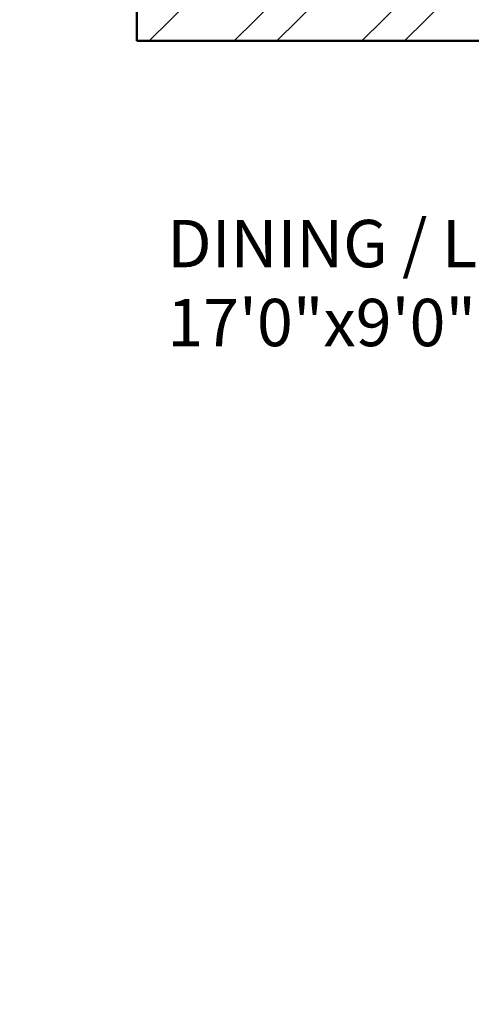
# Model space of a CAD drawing. Units: inches. Extents: x 963 to 2075, y 289 to 2657.
# Tile 89 of 98: x 1681 to 1728, y 2221 to 2325. Entities that reach past the tile are written whole.
import ezdxf

# ---------------------------------------------------------------- set-up
doc = ezdxf.new("R2010")
doc.units = ezdxf.units.IN
for name, color, linetype, lineweight in [('A-AREA-IDEN', 7, 'Continuous', 18), ('A-WALL', 7, 'Continuous', 50), ('A-WALL-PATT', 8, 'Continuous', 13)]:
    doc.layers.add(name, color=color, linetype=linetype, lineweight=lineweight)
doc.styles.get("Standard").update_dxf_attribs({"font": 'arial.ttf'})

msp = doc.modelspace()

# ---------------------------------------------------------------- hatches: boundary and pattern name
at = {"layer": 'A-WALL-PATT'}
h = msp.add_hatch(dxfattribs=at)
h.set_pattern_fill('ANSI32', color=256)
h.paths.add_polyline_path([(1296.92, 2558.32), (1203.92, 2558.32), (1203.92, 2493.82), (1191.53, 2493.82), (1191.53, 2489.32), (1211.06, 2489.32), (1211.06, 2492.02), (1211.06, 2493.82), (1208.42, 2493.82), (1208.42, 2553.82), (1292.42, 2553.82), (1292.42, 2538.86), (1296.92, 2538.86)])
h.paths.add_polyline_path([(1442.42, 2558.32), (1349.42, 2558.32), (1349.42, 2538.94), (1353.92, 2538.94), (1353.92, 2553.82), (1437.92, 2553.82), (1437.92, 2493.82), (1434.54, 2493.82), (1434.54, 2489.32), (1448.31, 2489.32), (1448.31, 2491.57), (1448.31, 2493.82), (1442.42, 2493.82)])
h.paths.add_polyline_path([(1415.55, 2491.57), (1415.55, 2493.82), (1340.94, 2493.82), (1340.94, 2489.32), (1371.92, 2489.32), (1371.92, 2378.32), (1367.6, 2378.32), (1367.6, 2373.82), (1371.92, 2373.82), (1371.92, 2355.19), (1376.42, 2355.19), (1376.42, 2489.32), (1415.55, 2489.32)])
h.paths.add_polyline_path([(1304.94, 2491.57), (1304.94, 2493.82), (1296.92, 2493.82), (1296.92, 2514.86), (1292.42, 2514.86), (1292.42, 2493.82), (1232.81, 2493.82), (1232.81, 2489.32), (1256.42, 2489.32), (1256.42, 2327.32), (1253.71, 2327.32), (1253.71, 2322.82), (1328.42, 2322.82), (1328.42, 2331.15), (1323.92, 2331.15), (1323.92, 2327.32), (1260.92, 2327.32), (1260.92, 2373.82), (1323.92, 2373.82), (1323.92, 2357.81), (1328.42, 2357.81), (1328.42, 2373.82), (1346.01, 2373.82), (1346.01, 2376.07), (1346.01, 2378.32), (1260.92, 2378.32), (1260.92, 2489.32), (1304.94, 2489.32)])
h.paths.add_polyline_path([(1226.65, 2327.32), (1124.42, 2327.32), (1124.42, 2347.45), (1119.92, 2347.45), (1119.92, 2322.82), (1163.42, 2322.82), (1163.42, 2305.43), (1165.67, 2305.43), (1167.92, 2305.43), (1167.92, 2322.82), (1226.65, 2322.82), (1226.65, 2325.07)])
h.paths.add_polyline_path([(1095.92, 2489.32), (1124.42, 2489.32), (1131.53, 2489.32), (1131.53, 2491.57), (1131.53, 2493.82), (1119.92, 2493.82), (1091.42, 2493.82), (1091.42, 2417.32), (1095.92, 2417.32), (1119.92, 2417.32), (1119.92, 2407.45), (1124.42, 2407.45), (1124.42, 2421.82), (1095.92, 2421.82)])
h.paths.add_polyline_path([(1512.92, 2558.32), (1508.42, 2558.32), (1508.42, 2493.82), (1503.4, 2493.82), (1503.4, 2489.32), (1508.42, 2489.32), (1508.42, 2327.32), (1376.42, 2327.32), (1376.42, 2330.27), (1371.92, 2330.27), (1371.92, 2298.74), (1376.42, 2298.74), (1376.42, 2322.82), (1508.42, 2322.82), (1508.42, 2165.32), (1504.26, 2165.32), (1504.26, 2160.82), (1508.42, 2160.82), (1508.42, 2108.32), (1512.92, 2108.32), (1512.92, 2160.82), (1516.18, 2160.82), (1516.18, 2163.07), (1516.18, 2165.32), (1512.92, 2165.32), (1512.92, 2322.82), (1644.92, 2322.82), (1644.92, 2298.74), (1649.42, 2298.74), (1649.42, 2322.82), (1649.42, 2330.94), (1647.17, 2330.94), (1644.92, 2330.94), (1644.92, 2327.32), (1512.92, 2327.32), (1512.92, 2489.32), (1516.76, 2489.32), (1516.76, 2491.57), (1516.76, 2493.82), (1512.92, 2493.82)])
h.paths.add_polyline_path([(1671.92, 2558.32), (1578.92, 2558.32), (1578.92, 2493.82), (1573.53, 2493.82), (1573.53, 2489.32), (1586.54, 2489.32), (1586.54, 2491.57), (1586.54, 2493.82), (1583.42, 2493.82), (1583.42, 2553.82), (1667.42, 2553.82), (1667.42, 2541.11), (1671.92, 2541.11)])
h.paths.add_polyline_path([(1681.26, 2493.82), (1671.92, 2493.82), (1671.92, 2517.11), (1667.42, 2517.11), (1667.42, 2493.82), (1610.22, 2493.82), (1610.22, 2489.32), (1644.92, 2489.32), (1644.92, 2357.87), (1649.42, 2357.87), (1649.42, 2373.82), (1652.2, 2373.82), (1652.2, 2375.83), (1652.2, 2378.32), (1649.42, 2378.32), (1649.42, 2489.32), (1681.26, 2489.32), (1681.26, 2491.57)])
h.paths.add_polyline_path([(1821.92, 2558.32), (1728.92, 2558.32), (1728.92, 2541), (1733.42, 2541), (1733.42, 2553.82), (1817.42, 2553.82), (1817.42, 2493.82), (1813.51, 2493.82), (1813.51, 2489.32), (1830.08, 2489.32), (1830.08, 2491.57), (1830.08, 2493.82), (1821.92, 2493.82)])
h.paths.add_polyline_path([(1794.24, 2493.82), (1717.26, 2493.82), (1717.26, 2489.32), (1760.42, 2489.32), (1760.42, 2378.32), (1674.4, 2378.32), (1674.4, 2373.82), (1692.92, 2373.82), (1692.92, 2356.95), (1697.42, 2356.95), (1697.42, 2373.82), (1760.42, 2373.82), (1760.42, 2327.32), (1697.42, 2327.32), (1697.42, 2333.34), (1692.92, 2333.34), (1692.92, 2322.82), (1768.04, 2322.82), (1768.04, 2325.07), (1768.04, 2327.32), (1764.92, 2327.32), (1764.92, 2489.32), (1794.24, 2489.32)])
h.paths.add_polyline_path([(1733.42, 2517), (1728.92, 2517), (1728.92, 2493.82), (1733.42, 2493.82)], flags=17)
h.paths.add_polyline_path([(1929.92, 2493.82), (1890.08, 2493.82), (1890.08, 2489.32), (1896.92, 2489.32), (1925.42, 2489.32), (1925.42, 2421.82), (1896.92, 2421.82), (1896.92, 2408.32), (1901.42, 2408.32), (1901.42, 2417.32), (1925.42, 2417.32), (1929.92, 2417.32)])
h.paths.add_polyline_path([(1901.42, 2348.32), (1896.92, 2348.32), (1896.92, 2327.32), (1800.42, 2327.32), (1800.42, 2322.82), (1853.42, 2322.82), (1853.42, 2309.45), (1857.92, 2309.45), (1857.92, 2322.82), (1901.42, 2322.82)])
h.paths.add_polyline_path([(1857.92, 2249.45), (1853.42, 2249.45), (1853.42, 2214.82), (1686.31, 2214.82), (1686.31, 2210.32), (1853.42, 2210.32), (1853.42, 2202.13), (1857.92, 2202.13), (1857.92, 2210.32)])
h.paths.add_polyline_path([(1857.92, 2142.13), (1853.42, 2142.13), (1853.42, 2115.42), (1841.42, 2115.42), (1841.42, 2088.53), (1841.42, 2046.95), (1845.92, 2046.95), (1845.92, 2110.92), (1905.92, 2110.92), (1905.92, 2092.52), (1910.42, 2092.52), (1910.42, 2115.42), (1857.92, 2115.42)])
h.paths.add_polyline_path([(1532.44, 1482.34), (1573.46, 1482.34), (1573.46, 1501), (1532.44, 1501)], flags=9)
h.paths.add_polyline_path([(1438.66, 1486.3), (1479.68, 1486.3), (1479.68, 1504.96), (1438.66, 1504.96)], flags=9)
h.paths.add_polyline_path([(1411.22, 1365.31), (1659.14, 1365.31), (1659.14, 1402.4), (1411.22, 1402.4)], flags=9)
h.paths.add_polyline_path([(1185.67, 2296.3), (1248.16, 2296.3), (1248.16, 2314.95), (1185.67, 2314.95)], flags=9)
h.paths.add_polyline_path([(1177.31, 2187.35), (1216.15, 2187.35), (1216.15, 2206.01), (1177.31, 2206.01)], flags=9)
h.paths.add_polyline_path([(1295.1, 1602.08), (1328.26, 1602.08), (1328.26, 1620.74), (1295.1, 1620.74)], flags=9)
h.paths.add_polyline_path([(1525.13, 2005.99), (1558.39, 2005.99), (1558.39, 2024.65), (1525.13, 2024.65)], flags=9)
h.paths.add_polyline_path([(1459.61, 1977.13), (1472.19, 1977.13), (1472.19, 1987.43), (1459.61, 1987.43)], flags=9)
h.paths.add_polyline_path([(1467.81, 2053.68), (1480.02, 2053.68), (1480.02, 2063.98), (1467.81, 2063.98)], flags=9)
h.paths.add_polyline_path([(1555.18, 2119.02), (1584.56, 2119.02), (1584.56, 2137.68), (1555.18, 2137.68)], flags=25)
h.paths.add_polyline_path([(1405.39, 2115.29), (1444.48, 2115.29), (1444.48, 2133.95), (1405.39, 2133.95)], flags=25)
h.paths.add_polyline_path([(1698.48, 2004.26), (1727.69, 2004.26), (1727.69, 2022.92), (1698.48, 2022.92)], flags=9)
h.paths.add_polyline_path([(1612.16, 1972.86), (1629.02, 1972.86), (1629.02, 1983.16), (1612.16, 1983.16)], flags=9)
h.paths.add_polyline_path([(1608.29, 2060.04), (1625.15, 2060.04), (1625.15, 2070.34), (1608.29, 2070.34)], flags=9)
h.paths.add_polyline_path([(1527.95, 1684.4), (1566.79, 1684.4), (1566.79, 1703.06), (1527.95, 1703.06)], flags=9)
h.paths.add_polyline_path([(1422.79, 1683.59), (1461.63, 1683.59), (1461.63, 1702.25), (1422.79, 1702.25)], flags=9)
h.paths.add_polyline_path([(1531.26, 1732.46), (1574.01, 1732.46), (1574.01, 1751.12), (1531.26, 1751.12)], flags=9)
h.paths.add_polyline_path([(1402.87, 1732.85), (1439.8, 1732.85), (1439.8, 1751.5), (1402.87, 1751.5)], flags=9)
h.paths.add_polyline_path([(1243.12, 1923.13), (1281.96, 1923.13), (1281.96, 1941.79), (1243.12, 1941.79)], flags=9)
h.paths.add_polyline_path([(1181.75, 1792.27), (1244.24, 1792.27), (1244.24, 1810.93), (1181.75, 1810.93)], flags=9)
h.paths.add_polyline_path([(1265.82, 1670.3), (1316.07, 1670.3), (1316.07, 1688.96), (1265.82, 1688.96)], flags=9)
h.paths.add_polyline_path([(1140.26, 1676.05), (1179.1, 1676.05), (1179.1, 1694.71), (1140.26, 1694.71)], flags=9)
h.paths.add_polyline_path([(1107.49, 1490.89), (1143.37, 1490.89), (1143.37, 1509.55), (1107.49, 1509.55)], flags=9)
h.paths.add_polyline_path([(1217.58, 1483.9), (1246.74, 1483.9), (1246.74, 1502.56), (1217.58, 1502.56)], flags=9)
h.paths.add_polyline_path([(1389.21, 1486.92), (1418.37, 1486.92), (1418.37, 1505.58), (1389.21, 1505.58)], flags=9)
h.paths.add_polyline_path([(1672.21, 1602.08), (1705.37, 1602.08), (1705.37, 1620.74), (1672.21, 1620.74)], flags=9)
h.paths.add_polyline_path([(1752.08, 1522.64), (1781.24, 1522.64), (1781.24, 1541.3), (1752.08, 1541.3)], flags=9)
h.paths.add_polyline_path([(1848.27, 1491.26), (1884.16, 1491.26), (1884.16, 1509.92), (1848.27, 1509.92)], flags=9)
h.paths.add_polyline_path([(1822.47, 1685.62), (1861.31, 1685.62), (1861.31, 1704.28), (1822.47, 1704.28)], flags=9)
h.paths.add_polyline_path([(1713.19, 1672.23), (1763.44, 1672.23), (1763.44, 1690.89), (1713.19, 1690.89)], flags=9)
h.paths.add_polyline_path([(1736.62, 1790.58), (1799.11, 1790.58), (1799.11, 1809.24), (1736.62, 1809.24)], flags=9)
h.paths.add_polyline_path([(1691.49, 1916.36), (1730.33, 1916.36), (1730.33, 1935.01), (1691.49, 1935.01)], flags=9)
h.paths.add_polyline_path([(1764.87, 1973.92), (1794.31, 1973.92), (1794.31, 1992.58), (1764.87, 1992.58)], flags=9)
h.paths.add_polyline_path([(1767.85, 2034.02), (1797.29, 2034.02), (1797.29, 2052.67), (1767.85, 2052.67)], flags=9)
h.paths.add_polyline_path([(1851.59, 2060.33), (1880.75, 2060.33), (1880.75, 2078.99), (1851.59, 2078.99)], flags=25)
h.paths.add_polyline_path([(1688.49, 2086.87), (1727.33, 2086.87), (1727.33, 2105.53), (1688.49, 2105.53)], flags=9)
h.paths.add_polyline_path([(1537.74, 2293.58), (1580.49, 2293.58), (1580.49, 2312.24), (1537.74, 2312.24)], flags=25)
h.paths.add_polyline_path([(1425.59, 2296.11), (1468.34, 2296.11), (1468.34, 2314.77), (1425.59, 2314.77)], flags=25)
h.paths.add_polyline_path([(1278.52, 2004.18), (1307.72, 2004.18), (1307.72, 2022.84), (1278.52, 2022.84)], flags=9)
h.paths.add_polyline_path([(1193.28, 1973.63), (1222.72, 1973.63), (1222.72, 1992.29), (1193.28, 1992.29)], flags=9)
h.paths.add_polyline_path([(1192.41, 2040.58), (1221.84, 2040.58), (1221.84, 2059.23), (1192.41, 2059.23)], flags=9)
h.paths.add_polyline_path([(1130.6, 1951.39), (1159.76, 1951.39), (1159.76, 1970.05), (1130.6, 1970.05)], flags=9)
h.paths.add_polyline_path([(1132.83, 2052.49), (1161.98, 2052.49), (1161.98, 2071.15), (1132.83, 2071.15)], flags=9)
h.paths.add_polyline_path([(1265.13, 2334.62), (1315.38, 2334.62), (1315.38, 2353.28), (1265.13, 2353.28)], flags=25)
h.paths.add_polyline_path([(1136.74, 2330.79), (1175.58, 2330.79), (1175.58, 2349.44), (1136.74, 2349.44)], flags=9)
h.paths.add_polyline_path([(1287.42, 2417.2), (1320.58, 2417.2), (1320.58, 2435.86), (1287.42, 2435.86)], flags=25)
h.paths.add_polyline_path([(1430.99, 2329.16), (1469.83, 2329.16), (1469.83, 2347.82), (1430.99, 2347.82)], flags=25)
h.paths.add_polyline_path([(1525.42, 2329.21), (1564.26, 2329.21), (1564.26, 2347.87), (1525.42, 2347.87)], flags=25)
h.paths.add_polyline_path([(1684.52, 2382.8), (1717.68, 2382.8), (1717.68, 2401.46), (1684.52, 2401.46)], flags=25)
h.paths.add_polyline_path([(1704.81, 2340.29), (1755.05, 2340.29), (1755.05, 2358.95), (1704.81, 2358.95)], flags=25)
h.paths.add_polyline_path([(1694.11, 2287.76), (1756.6, 2287.76), (1756.6, 2306.41), (1694.11, 2306.41)], flags=9)
h.paths.add_polyline_path([(1815.78, 2329.86), (1854.62, 2329.86), (1854.62, 2348.52), (1815.78, 2348.52)], flags=9)
h.paths.add_polyline_path([(1842.87, 2514.26), (1878.76, 2514.26), (1878.76, 2532.91), (1842.87, 2532.91)], flags=9)
h.paths.add_polyline_path([(1769.51, 2531.45), (1798.67, 2531.45), (1798.67, 2550.1), (1769.51, 2550.1)], flags=25)
h.paths.add_polyline_path([(1594.77, 2518.47), (1623.93, 2518.47), (1623.93, 2537.13), (1594.77, 2537.13)], flags=25)
h.paths.add_polyline_path([(1520.72, 2516.18), (1556.61, 2516.18), (1556.61, 2534.84), (1520.72, 2534.84)], flags=25)
h.paths.add_polyline_path([(1464.46, 2516.69), (1500.34, 2516.69), (1500.34, 2535.35), (1464.46, 2535.35)], flags=25)
h.paths.add_polyline_path([(1365.7, 2528.97), (1394.85, 2528.97), (1394.85, 2547.63), (1365.7, 2547.63)], flags=25)
h.paths.add_polyline_path([(1222.84, 2516.23), (1252, 2516.23), (1252, 2534.89), (1222.84, 2534.89)], flags=25)
h.paths.add_polyline_path([(1104.55, 2509.6), (1140.43, 2509.6), (1140.43, 2528.26), (1104.55, 2528.26)], flags=9)
h = msp.add_hatch(dxfattribs=at)
h.set_pattern_fill('ANSI32', color=256)
h.paths.add_polyline_path([(1335.97, 2212.57), (1335.97, 2214.82), (1167.92, 2214.82), (1167.92, 2245.43), (1163.42, 2245.43), (1163.42, 2210.32), (1163.42, 2194.81), (1167.92, 2194.81), (1167.92, 2210.32), (1335.97, 2210.32)])
h.paths.add_polyline_path([(1532.44, 1482.34), (1573.46, 1482.34), (1573.46, 1501), (1532.44, 1501)], flags=9)
h.paths.add_polyline_path([(1438.66, 1486.3), (1479.68, 1486.3), (1479.68, 1504.96), (1438.66, 1504.96)], flags=9)
h.paths.add_polyline_path([(1411.22, 1365.31), (1659.14, 1365.31), (1659.14, 1402.4), (1411.22, 1402.4)], flags=9)
h.paths.add_polyline_path([(1185.67, 2296.3), (1248.16, 2296.3), (1248.16, 2314.95), (1185.67, 2314.95)], flags=9)
h.paths.add_polyline_path([(1177.31, 2187.35), (1216.15, 2187.35), (1216.15, 2206.01), (1177.31, 2206.01)], flags=9)
h.paths.add_polyline_path([(1295.1, 1602.08), (1328.26, 1602.08), (1328.26, 1620.74), (1295.1, 1620.74)], flags=9)
h.paths.add_polyline_path([(1525.13, 2005.99), (1558.39, 2005.99), (1558.39, 2024.65), (1525.13, 2024.65)], flags=9)
h.paths.add_polyline_path([(1459.61, 1977.13), (1472.19, 1977.13), (1472.19, 1987.43), (1459.61, 1987.43)], flags=9)
h.paths.add_polyline_path([(1467.81, 2053.68), (1480.02, 2053.68), (1480.02, 2063.98), (1467.81, 2063.98)], flags=9)
h.paths.add_polyline_path([(1555.18, 2119.02), (1584.56, 2119.02), (1584.56, 2137.68), (1555.18, 2137.68)], flags=9)
h.paths.add_polyline_path([(1405.39, 2115.29), (1444.48, 2115.29), (1444.48, 2133.95), (1405.39, 2133.95)], flags=9)
h.paths.add_polyline_path([(1698.48, 2004.26), (1727.69, 2004.26), (1727.69, 2022.92), (1698.48, 2022.92)], flags=9)
h.paths.add_polyline_path([(1612.16, 1972.86), (1629.02, 1972.86), (1629.02, 1983.16), (1612.16, 1983.16)], flags=9)
h.paths.add_polyline_path([(1608.29, 2060.04), (1625.15, 2060.04), (1625.15, 2070.34), (1608.29, 2070.34)], flags=9)
h.paths.add_polyline_path([(1527.95, 1684.4), (1566.79, 1684.4), (1566.79, 1703.06), (1527.95, 1703.06)], flags=9)
h.paths.add_polyline_path([(1422.79, 1683.59), (1461.63, 1683.59), (1461.63, 1702.25), (1422.79, 1702.25)], flags=9)
h.paths.add_polyline_path([(1531.26, 1732.46), (1574.01, 1732.46), (1574.01, 1751.12), (1531.26, 1751.12)], flags=9)
h.paths.add_polyline_path([(1402.87, 1732.85), (1439.8, 1732.85), (1439.8, 1751.5), (1402.87, 1751.5)], flags=9)
h.paths.add_polyline_path([(1243.12, 1923.13), (1281.96, 1923.13), (1281.96, 1941.79), (1243.12, 1941.79)], flags=9)
h.paths.add_polyline_path([(1181.75, 1792.27), (1244.24, 1792.27), (1244.24, 1810.93), (1181.75, 1810.93)], flags=9)
h.paths.add_polyline_path([(1265.82, 1670.3), (1316.07, 1670.3), (1316.07, 1688.96), (1265.82, 1688.96)], flags=9)
h.paths.add_polyline_path([(1140.26, 1676.05), (1179.1, 1676.05), (1179.1, 1694.71), (1140.26, 1694.71)], flags=9)
h.paths.add_polyline_path([(1107.49, 1490.89), (1143.37, 1490.89), (1143.37, 1509.55), (1107.49, 1509.55)], flags=9)
h.paths.add_polyline_path([(1217.58, 1483.9), (1246.74, 1483.9), (1246.74, 1502.56), (1217.58, 1502.56)], flags=9)
h.paths.add_polyline_path([(1389.21, 1486.92), (1418.37, 1486.92), (1418.37, 1505.58), (1389.21, 1505.58)], flags=9)
h.paths.add_polyline_path([(1672.21, 1602.08), (1705.37, 1602.08), (1705.37, 1620.74), (1672.21, 1620.74)], flags=9)
h.paths.add_polyline_path([(1752.08, 1522.64), (1781.24, 1522.64), (1781.24, 1541.3), (1752.08, 1541.3)], flags=9)
h.paths.add_polyline_path([(1848.27, 1491.26), (1884.16, 1491.26), (1884.16, 1509.92), (1848.27, 1509.92)], flags=9)
h.paths.add_polyline_path([(1822.47, 1685.62), (1861.31, 1685.62), (1861.31, 1704.28), (1822.47, 1704.28)], flags=9)
h.paths.add_polyline_path([(1713.19, 1672.23), (1763.44, 1672.23), (1763.44, 1690.89), (1713.19, 1690.89)], flags=9)
h.paths.add_polyline_path([(1736.62, 1790.58), (1799.11, 1790.58), (1799.11, 1809.24), (1736.62, 1809.24)], flags=9)
h.paths.add_polyline_path([(1691.49, 1916.36), (1730.33, 1916.36), (1730.33, 1935.01), (1691.49, 1935.01)], flags=9)
h.paths.add_polyline_path([(1764.87, 1973.92), (1794.31, 1973.92), (1794.31, 1992.58), (1764.87, 1992.58)], flags=9)
h.paths.add_polyline_path([(1767.85, 2034.02), (1797.29, 2034.02), (1797.29, 2052.67), (1767.85, 2052.67)], flags=9)
h.paths.add_polyline_path([(1851.59, 2060.33), (1880.75, 2060.33), (1880.75, 2078.99), (1851.59, 2078.99)], flags=9)
h.paths.add_polyline_path([(1688.49, 2086.87), (1727.33, 2086.87), (1727.33, 2105.53), (1688.49, 2105.53)], flags=9)
h.paths.add_polyline_path([(1537.74, 2293.58), (1580.49, 2293.58), (1580.49, 2312.24), (1537.74, 2312.24)], flags=9)
h.paths.add_polyline_path([(1425.59, 2296.11), (1468.34, 2296.11), (1468.34, 2314.77), (1425.59, 2314.77)], flags=9)
h.paths.add_polyline_path([(1278.52, 2004.18), (1307.72, 2004.18), (1307.72, 2022.84), (1278.52, 2022.84)], flags=9)
h.paths.add_polyline_path([(1193.28, 1973.63), (1222.72, 1973.63), (1222.72, 1992.29), (1193.28, 1992.29)], flags=9)
h.paths.add_polyline_path([(1192.41, 2040.58), (1221.84, 2040.58), (1221.84, 2059.23), (1192.41, 2059.23)], flags=9)
h.paths.add_polyline_path([(1130.6, 1951.39), (1159.76, 1951.39), (1159.76, 1970.05), (1130.6, 1970.05)], flags=9)
h.paths.add_polyline_path([(1132.83, 2052.49), (1161.98, 2052.49), (1161.98, 2071.15), (1132.83, 2071.15)], flags=9)
h.paths.add_polyline_path([(1265.13, 2334.62), (1315.38, 2334.62), (1315.38, 2353.28), (1265.13, 2353.28)], flags=9)
h.paths.add_polyline_path([(1136.74, 2330.79), (1175.58, 2330.79), (1175.58, 2349.44), (1136.74, 2349.44)], flags=9)
h.paths.add_polyline_path([(1287.42, 2417.2), (1320.58, 2417.2), (1320.58, 2435.86), (1287.42, 2435.86)], flags=9)
h.paths.add_polyline_path([(1430.99, 2329.16), (1469.83, 2329.16), (1469.83, 2347.82), (1430.99, 2347.82)], flags=9)
h.paths.add_polyline_path([(1525.42, 2329.21), (1564.26, 2329.21), (1564.26, 2347.87), (1525.42, 2347.87)], flags=9)
h.paths.add_polyline_path([(1684.52, 2382.8), (1717.68, 2382.8), (1717.68, 2401.46), (1684.52, 2401.46)], flags=9)
h.paths.add_polyline_path([(1704.81, 2340.29), (1755.05, 2340.29), (1755.05, 2358.95), (1704.81, 2358.95)], flags=9)
h.paths.add_polyline_path([(1694.11, 2287.76), (1756.6, 2287.76), (1756.6, 2306.41), (1694.11, 2306.41)], flags=9)
h.paths.add_polyline_path([(1815.78, 2329.86), (1854.62, 2329.86), (1854.62, 2348.52), (1815.78, 2348.52)], flags=9)
h.paths.add_polyline_path([(1842.87, 2514.26), (1878.76, 2514.26), (1878.76, 2532.91), (1842.87, 2532.91)], flags=9)
h.paths.add_polyline_path([(1769.51, 2531.45), (1798.67, 2531.45), (1798.67, 2550.1), (1769.51, 2550.1)], flags=9)
h.paths.add_polyline_path([(1594.77, 2518.47), (1623.93, 2518.47), (1623.93, 2537.13), (1594.77, 2537.13)], flags=9)
h.paths.add_polyline_path([(1520.72, 2516.18), (1556.61, 2516.18), (1556.61, 2534.84), (1520.72, 2534.84)], flags=9)
h.paths.add_polyline_path([(1464.46, 2516.69), (1500.34, 2516.69), (1500.34, 2535.35), (1464.46, 2535.35)], flags=9)
h.paths.add_polyline_path([(1365.7, 2528.97), (1394.85, 2528.97), (1394.85, 2547.63), (1365.7, 2547.63)], flags=9)
h.paths.add_polyline_path([(1222.84, 2516.23), (1252, 2516.23), (1252, 2534.89), (1222.84, 2534.89)], flags=9)
h.paths.add_polyline_path([(1104.55, 2509.6), (1140.43, 2509.6), (1140.43, 2528.26), (1104.55, 2528.26)], flags=9)

# ---------------------------------------------------------------- linework, layer by layer
at = {"layer": 'A-WALL'}
for p, q in [((1692.92, 2333.34), (1692.92, 2322.82)), ((1692.92, 2322.82), (1768.04, 2322.82))]:
    msp.add_line(p, q, dxfattribs=at)

# ---------------------------------------------------------------- texts
at = {"layer": 'A-AREA-IDEN', "insert": (1696.12, 2303.93), "char_height": 5, "attachment_point": 1}
msp.add_mtext_dynamic_manual_height_columns('DINING / LOUNGE\\P17\'0"x9\'0"', width=121.7947, gutter_width=12.5, heights=[0], dxfattribs=at)

doc.saveas('drawing.dxf')
